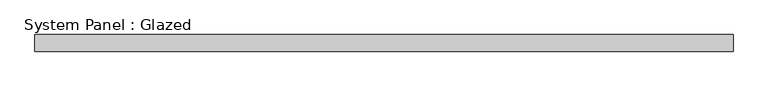
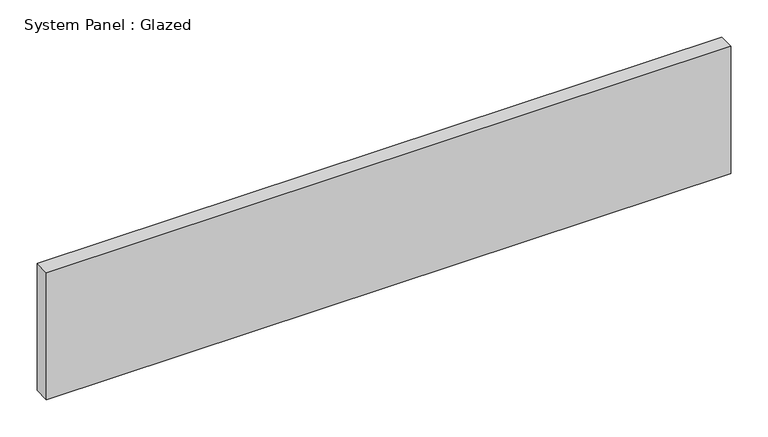
"""IFC4 building model written with IfcOpenShell, lengths in millimetres: plate geometry, System Panel : Glazed."""

from ifc_helpers import new_model, si_unit, origin, origin_with_axes, place, context, project, spatial, polyline, outline, extrude, source, transform, mapped, element, save


def system_panel_glazed_5a33b61e(model_context):
    return source(origin(), model_context, "Body", "SweptSolid", [
        extrude(outline(polyline([(533.4, 19.05), (-533.4, 19.05), (-533.4, 44.45), (533.4, 44.45), (533.4, 19.05)])), origin_with_axes(), (0.0, 0.0, 1.0), 209.55),
    ])


if __name__ == "__main__":
    model = new_model("IFC4")
    model_context = context("Model", 3, world=origin())
    ifc_project = project(units=[si_unit("LENGTHUNIT", "METRE", prefix="MILLI")], contexts=[model_context])
    site = spatial("IfcSite", under=ifc_project)
    building = spatial("IfcBuilding", under=site)
    placement = place(None, origin())
    system_panel_glazed_shape = system_panel_glazed_5a33b61e(model_context)
    element("IfcPlate", 1, ObjectType="System Panel : Glazed", at=placement, inside=building, context=model_context, shape_type="MappedRepresentation", body=[
        mapped(system_panel_glazed_shape, transform((0.0, 0.0, 0.0), x_axis=(1.0, 0.0, 0.0), y_axis=(0.0, 1.0, 0.0), z_axis=(0.0, 0.0, 1.0))),
    ])
    save(model, "model.ifc")

# Revit data of these elements
# Type "System Panel : Glazed"
#   Construction Type Id = "GSP4R"
#   Analytic Construction = "1/8 in Pilkington single glazing"
#   Visual Light Transmittance = 0.9
#   Solar Heat Gain Coefficient = 0.86
#   Heat Transfer Coefficient (U) = 1.18115 BTU/(h·ft²·°F)
#   Define Thermal Properties by = 1
# Element 1 (IfcPlate, "System Panel : Glazed")
#   Materials on its faces: "Glass"
# Materials
#   "Glass": class "Glass", colour RGB 0 128 192, transparency 0.75, Description = "Soda Lime Glass", Cost = 0
